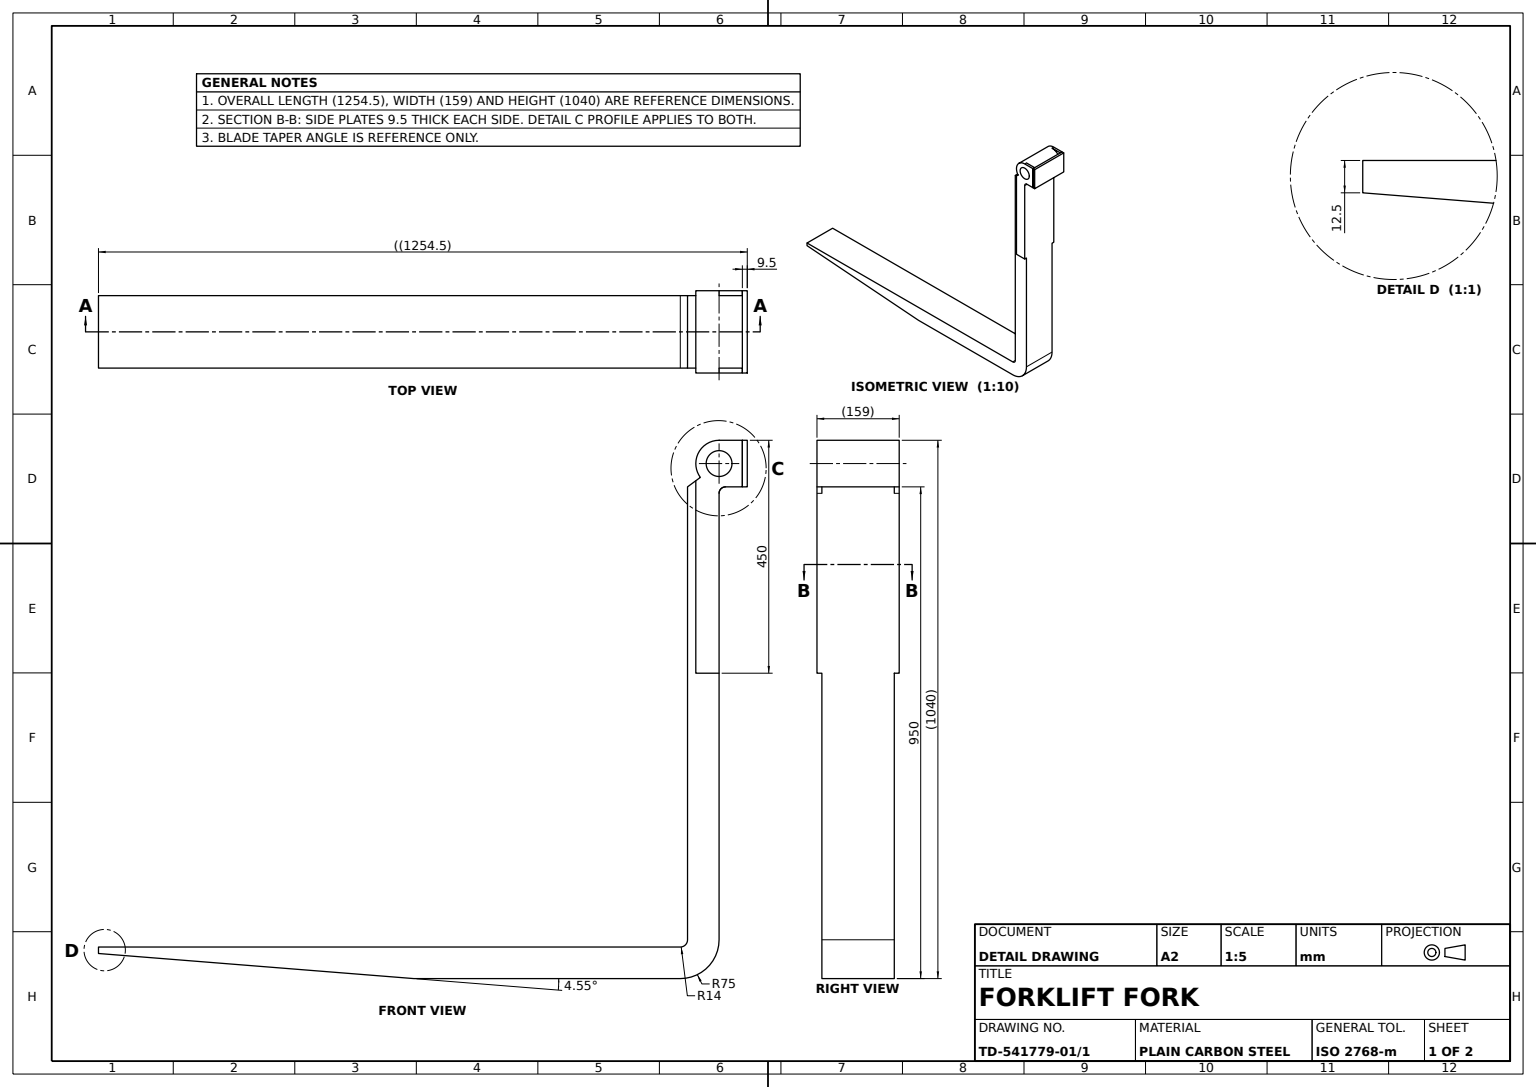
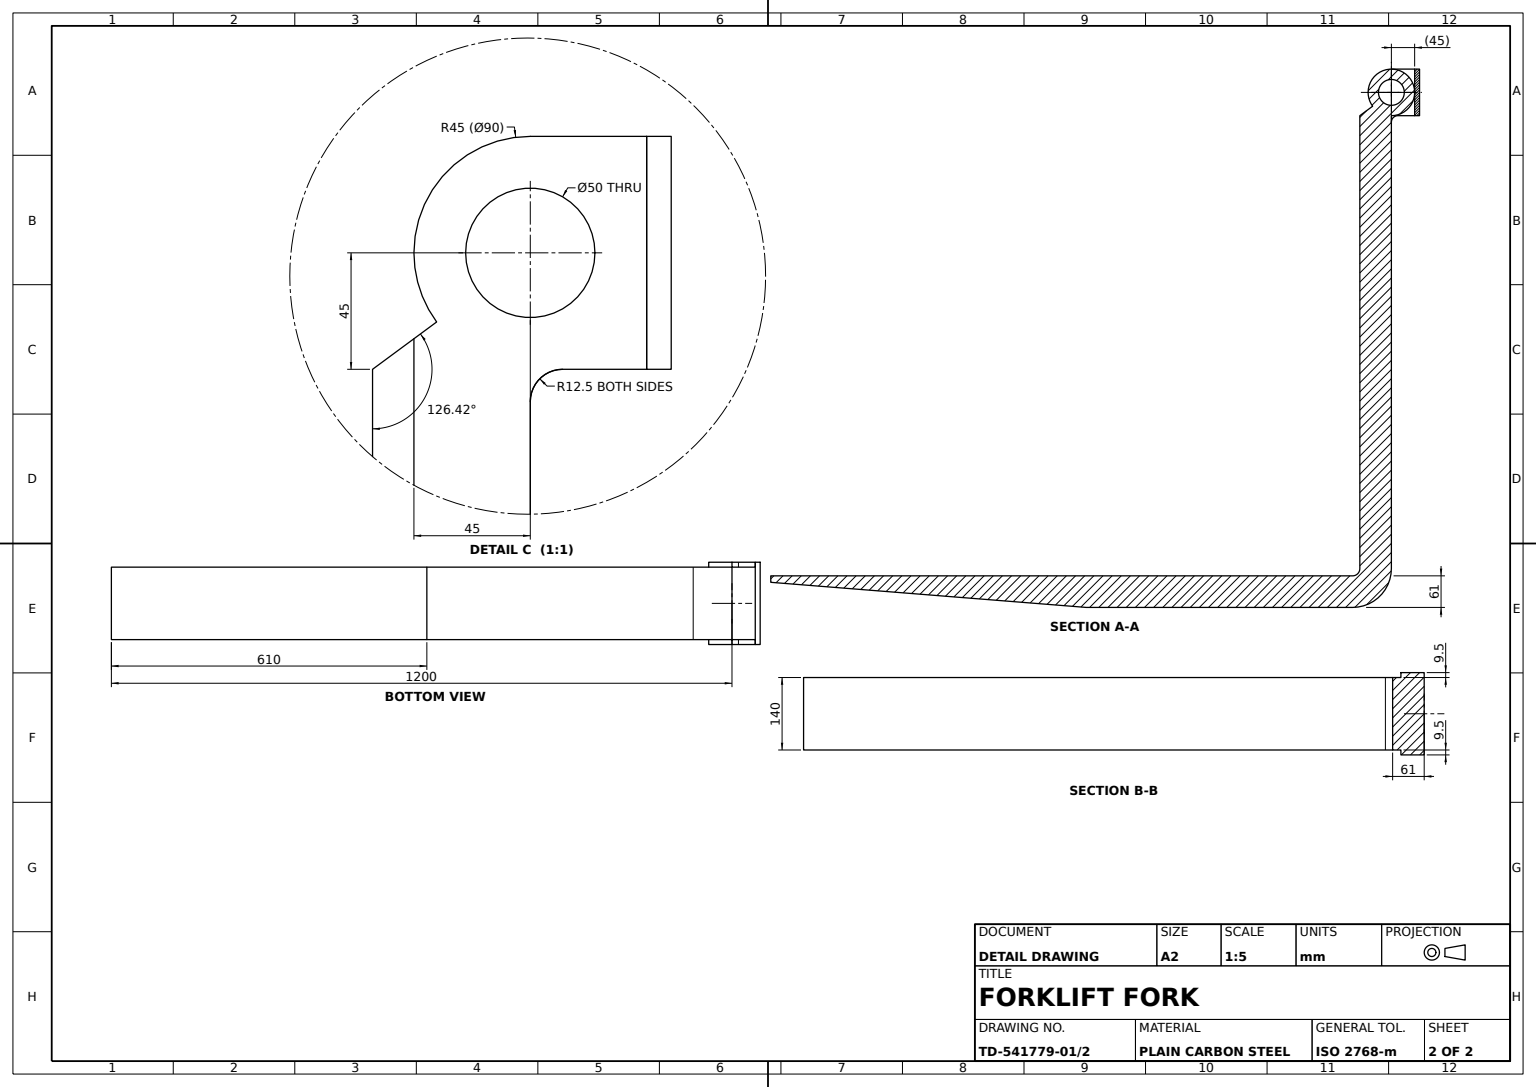
SolidWorks part; units mm, degrees
material "Plain Carbon Steel"
ref_plane "Front Plane" through (0, 0, 0) normal (0, 0, 1) x (1, 0, 0)
ref_plane "Top Plane" through (0, 0, 0) normal (0, 1, 0) x (1, 0, 0)
ref_plane "Right Plane" through (0, 0, 0) normal (1, 0, 0) x (0, 0, -1)
sketch "Fork L-Profile Sketch" plane through (0, 0, 0) normal (0, 0, 1) x (1, 0, 0)
  line L0 (0, 950) -> (0, 75)
  line L1 (-75, 0) -> (-1200, 0)
  arc A0 (0, 75) -> (-75, 0) centre (-75, 75) cw
  point P6 (0, 0)
  dimension "D3" = 75
  dimension "D1" = 1200
  dimension "D2" = 950
extrude "Fork Blade and Shank" add sketch "Fork L-Profile Sketch" along normal mid plane 140 thin
sketch "Blade Taper Sketch" plane through (0, 0, 70) normal (0, 0, 1) x (1, 0, 0)
  line L0 (-1200, 48.5) -> (-590, 0)
  line L1 (-1200, 0) -> (-1200, 61) construction
  line L2 (-75, 0) -> (-1200, 0) construction
  line L3 (-75, 61) -> (-1200, 61) construction
  dimension "D1" = 12.5
  dimension "D2" = 610
extrude "Blade Tip Taper Cut" cut sketch "Blade Taper Sketch" against normal through all both and the other way through all flip side to cut
sketch "Shank Boss Sketch" plane through (0, 0, 0) normal (0, 0, 1) x (1, 0, 0)
  line L0 (0, 950) -> (0, 1278.8206) construction
  circle A0 centre (0, 995) radius 45
  circle A1 centre (0, 995) radius 25
  dimension "D1" = 90
  dimension "D2" = 50
extrude "Shank Lower Boss" add sketch "Shank Boss Sketch" along normal mid plane 140 separate body contours A1 | A0
sketch "Shank Upper Boss Sketch" plane through (0, 0, 0) normal (0, 0, 1) x (1, 0, 0)
  line L0 (-61, 950) -> (0, 950) construction
  line L1 (-61, 950) -> (0, 950)
  line L2 (-61, 950) -> (-36.2126, 968.2858)
  circle A0 centre (0, 995) radius 45 construction
  circle A1 centre (0, 995) radius 45
extrude "Shank Upper Boss" add sketch "Shank Upper Boss Sketch" along normal mid plane 140 contours A1 L2 L1
sketch "Side Plate Sketch" plane through (0, 0, 70) normal (0, 0, 1) x (1, 0, 0)
  line L0 (-45, 995) -> (-45, 590)
  line L1 (0, 1040) -> (45, 1040)
  line L2 (45, 1040) -> (45, 950)
  line L3 (45, 950) -> (12.5, 950)
  line L4 (0, 950) -> (-61, 950)
  line L5 (0, 950) -> (0, 75) construction
  line L6 (0, 590) -> (-45, 590)
  line L7 (0, 937.5) -> (0, 590)
  arc A0 (0, 950) -> (-36.2126, 968.2858) centre (0, 995) ccw construction
  arc A2 (0, 937.5) -> (12.5, 950) centre (12.5, 937.5) cw
  arc A3 (-45, 995) -> (0, 1040) centre (0, 995) cw
  line M13 (0, 75) -> (0, 950)
  arc M14 (0, 950) -> (-36.2126, 968.2858) centre (0, 995) ccw
  line M15 (-36.2126, 968.2858) -> (-61, 950)
  circle M19 centre (0, 995) radius 25
  dimension "D1" = 12.5
  dimension "D2" = 45
  dimension "D3" = 450
extrude "Side Plate" add sketch "Side Plate Sketch" along normal blind 9.5 contours L2 L1 M14 | A2 L3 L2 M13 M14 | L4 L0 M14 M15 M19 | L6 L4 L0 M13
mirror "Side Plate Mirror" about plane through (0, 0, 0) normal (0, 0, 1) of "Side Plate"
sketch "Top Hook Block Sketch" plane through (45, 0, 0) normal (1, 0, 0) x (0, 0, -1)
  line L1 (-79.5, 1040) -> (79.5, 1040)
  line L2 (-79.5, 1040) -> (-79.5, 950)
  line L3 (-79.5, 950) -> (79.5, 950)
  line L4 (79.5, 1040) -> (79.5, 950)
extrude "Top Hook Block" add sketch "Top Hook Block Sketch" along normal blind 9.5 separate body
